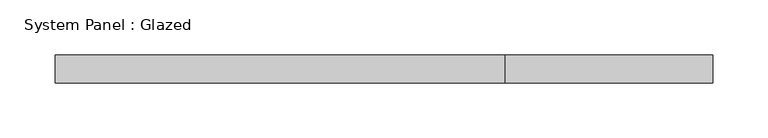
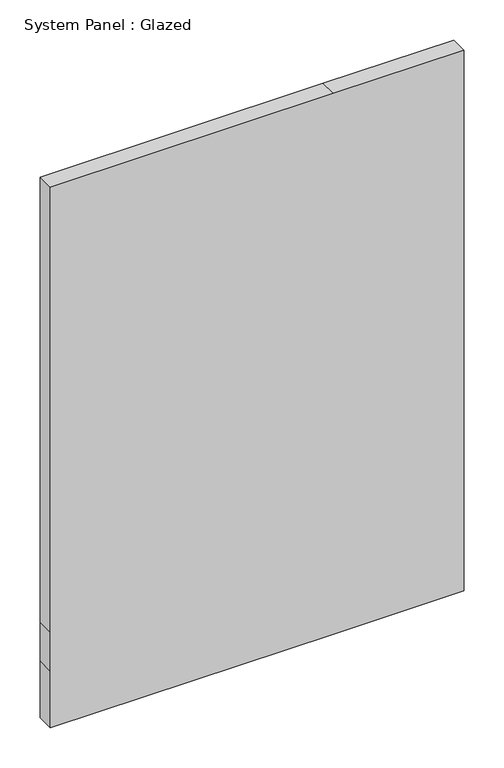
"""IFC4 building model written with IfcOpenShell, lengths in millimetres: plate geometry, System Panel : Glazed."""

from ifc_helpers import new_model, si_unit, frame, origin, place, context, project, spatial, polyline, outline, extrude, source, transform, mapped, element, save


def system_panel_glazed_a541dcfe(model_context):
    return source(origin(), model_context, "Body", "SweptSolid", [
        extrude(outline(polyline([(0.0, -298.45), (0.0, 110.0666667), (0.0, 298.45), (86.7833333, 298.45), (146.05, 298.45), (823.9658453, 298.45), (823.9658453, 110.0666667), (823.9658453, -298.45), (146.05, -298.45), (86.7833333, -298.45), (0.0, -298.45)])), frame((0.0, 19.05, 0.0), z_axis=(0.0, 1.0, 0.0), x_axis=(0.0, 0.0, 1.0)), (0.0, 0.0, 1.0), 25.4),
    ])


if __name__ == "__main__":
    model = new_model("IFC4")
    model_context = context("Model", 3, world=origin())
    ifc_project = project(units=[si_unit("LENGTHUNIT", "METRE", prefix="MILLI")], contexts=[model_context])
    site = spatial("IfcSite", under=ifc_project)
    building = spatial("IfcBuilding", under=site)
    placement = place(None, origin())
    system_panel_glazed_shape = system_panel_glazed_a541dcfe(model_context)
    element("IfcPlate", 1, ObjectType="System Panel : Glazed", at=placement, inside=building, context=model_context, shape_type="MappedRepresentation", body=[
        mapped(system_panel_glazed_shape, transform((0.0, 0.0, 0.0), x_axis=(1.0, 0.0, 0.0), y_axis=(0.0, 1.0, 0.0), z_axis=(0.0, 0.0, 1.0))),
    ])
    save(model, "model.ifc")

# Revit data of these elements
# Type "System Panel : Glazed"
#   Construction Type Id = "GSP4R"
#   Analytic Construction = "1/8 in Pilkington single glazing"
#   Visual Light Transmittance = 0.9
#   Solar Heat Gain Coefficient = 0.86
#   Heat Transfer Coefficient (U) = 1.18115 BTU/(h·ft²·°F)
#   Define Thermal Properties by = 1
# Element 1 (IfcPlate, "System Panel : Glazed")
#   Materials on its faces: "Glass"
# Materials
#   "Glass": class "Glass", colour RGB 0 128 192, transparency 0.75, Description = "Soda Lime Glass", Cost = 0
